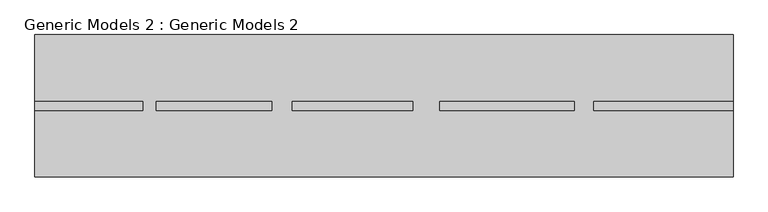
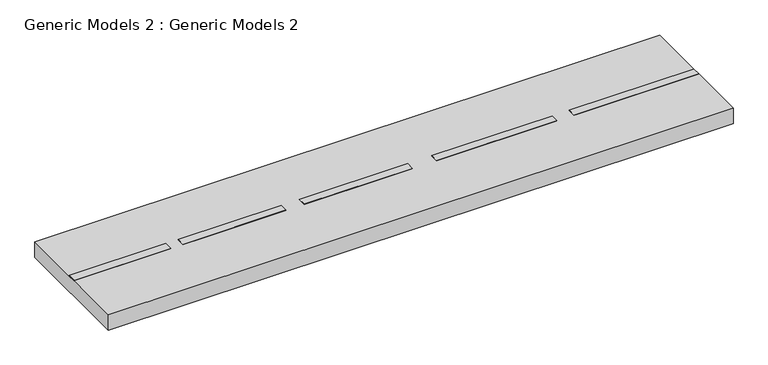
"""IFC4 building model written with IfcOpenShell, lengths in millimetres: proxy geometry, Generic Models 2 : Generic Models 2."""

from ifc_helpers import new_model, si_unit, frame, origin, origin_with_axes, place, context, project, spatial, polyline, outline, extrude, source, transform, mapped, element, save


def generic_models_2_generic_models_2_314bea4d(model_context):
    return source(origin(), model_context, "Body", "SweptSolid", [
        extrude(outline(polyline([(-7525.0794906, -9547.4142637), (-9953.4065481, -9547.4142637), (-9953.4065481, -9344.2142637), (-7525.0794906, -9344.2142637), (-7525.0794906, -9547.4142637)])), origin_with_axes(), (0.0, 0.0, 1.0), 12.0054688),
        extrude(outline(polyline([(5743.7934519, -9344.2142637), (5743.7934519, -9547.4142637), (2608.635938, -9547.4142637), (2608.635938, -9344.2142637), (5743.7934519, -9344.2142637)])), origin_with_axes(), (0.0, 0.0, 1.0), 12.0054688),
        extrude(outline(polyline([(-7220.2794906, -9344.2142637), (-4630.364062, -9344.2142637), (-4630.364062, -9547.4142637), (-7220.2794906, -9547.4142637), (-7220.2794906, -9344.2142637)])), origin_with_axes(), (0.0, 0.0, 1.0), 12.0054688),
        extrude(outline(polyline([(-4173.164062, -9344.2142637), (-1455.364062, -9344.2142637), (-1455.364062, -9547.4142637), (-4173.164062, -9547.4142637), (-4173.164062, -9344.2142637)])), origin_with_axes(), (0.0, 0.0, 1.0), 12.0054688),
        extrude(outline(polyline([(-845.764062, -9344.2142637), (2176.835938, -9344.2142637), (2176.835938, -9547.4142637), (-845.764062, -9547.4142637), (-845.764062, -9344.2142637)])), origin_with_axes(), (0.0, 0.0, 1.0), 12.0054688),
        extrude(outline(polyline([(5743.7934519, -7845.6142637), (5743.7934519, -11046.0142637), (-9953.4065481, -11046.0142637), (-9953.4065481, -7845.6142637), (5743.7934519, -7845.6142637)])), frame((0.0, 0.0, -406.4), z_axis=(0.0, 0.0, 1.0), x_axis=(1.0, 0.0, 0.0)), (0.0, 0.0, 1.0), 406.4),
    ])


if __name__ == "__main__":
    model = new_model("IFC4")
    model_context = context("Model", 3, world=origin())
    ifc_project = project(units=[si_unit("LENGTHUNIT", "METRE", prefix="MILLI")], contexts=[model_context])
    site = spatial("IfcSite", under=ifc_project)
    building = spatial("IfcBuilding", under=site)
    placement = place(None, origin())
    generic_models_2_generic_models_2_shape = generic_models_2_generic_models_2_314bea4d(model_context)
    element("IfcBuildingElementProxy", 1, Name="Generic Models 2 : Generic Models 2", ObjectType="Generic Models 2 : Generic Models 2", at=placement, inside=building, context=model_context, shape_type="MappedRepresentation", body=[
        mapped(generic_models_2_generic_models_2_shape, transform((0.0, 0.0, 0.0), x_axis=(1.0, 0.0, 0.0), y_axis=(0.0, 1.0, 0.0), z_axis=(0.0, 0.0, 1.0))),
    ])
    save(model, "model.ifc")

# Revit data of these elements
# Element 1 (IfcBuildingElementProxy, "Generic Models 2 : Generic Models 2")
#   Materials on its faces: "ROAD"
# Materials
#   "ROAD": class "Generic", colour RGB 120 120 120, transparency 0, Cost = 0
